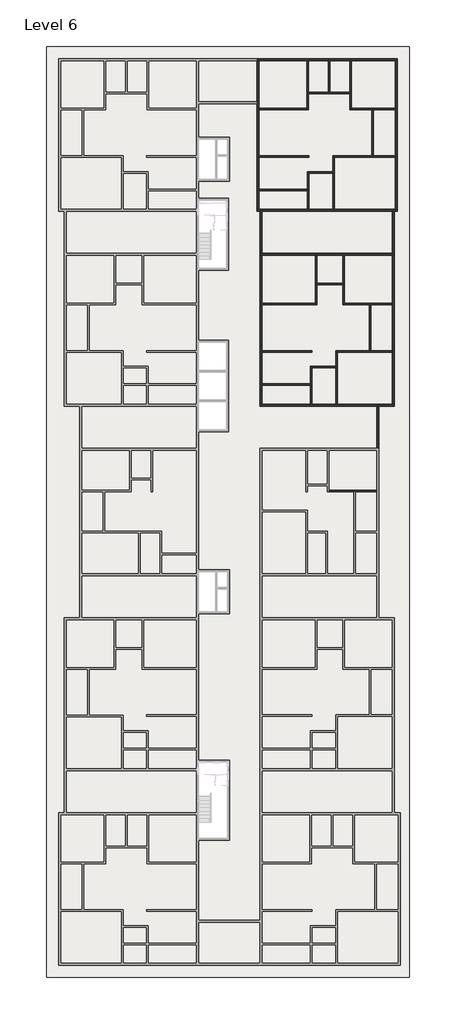
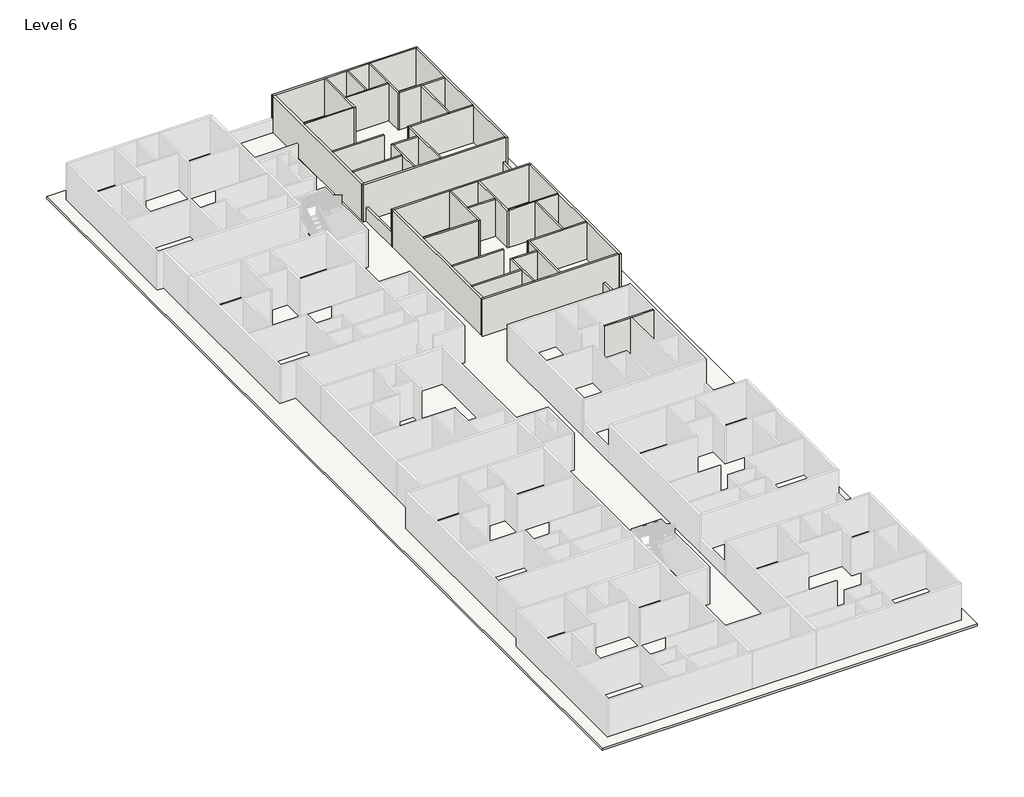
# One storey, part 4 of 8: 37 walls, 1 roof, 1 slab.
"""IFC4 building model written with IfcOpenShell, lengths in millimetres."""

from ifc_helpers import new_model, si_unit, frame, origin, place, context, project, spatial, polyline, outline, extrude, faceted_brep, element, save

model = new_model("IFC4")

# Units and contexts
model_context = context("Model", 3, world=origin())
ifc_project = project(units=[si_unit("LENGTHUNIT", "METRE", prefix="MILLI")], contexts=[model_context])

# Site, building, storey
site = spatial("IfcSite", under=ifc_project)
building = spatial("IfcBuilding", under=site)
storey = spatial("IfcBuildingStorey", under=building, Name="Level 6", Elevation=40474.6172466)

# Roof
placement = place(None, origin())
element("IfcRoof", 1, ObjectType="SLAB", at=placement, inside=storey, context=model_context, shape_type="SweptSolid", body=[
    extrude(outline(polyline([(-15237.9415084, -35021.5344126), (-15237.9415084, 36097.9216096), (12498.9443719, 36097.9216096), (12498.9443719, -35021.5344126), (-15237.9415084, -35021.5344126)]), holes=[polyline([(-3617.4415084, 29152.4900967), (-3617.4415084, 25799.6900967), (-1255.2415084, 25799.6900967), (-1255.2415084, 29152.4900967), (-3617.4415084, 29152.4900967)]), polyline([(-3617.4415084, 24490.1216096), (-3617.4415084, 19003.7216096), (-1331.4415084, 19003.7216096), (-1331.4415084, 24490.1216096), (-3617.4415084, 24490.1216096)]), polyline([(-3617.4415084, 13669.6303368), (-3617.4415084, 6659.2303368), (-1331.4415084, 6659.2303368), (-1331.4415084, 13669.6303368), (-3617.4415084, 13669.6303368)]), polyline([(-3617.4415084, -3882.2751812), (-3617.4415084, -7235.0751812), (-1255.2415084, -7235.0751812), (-1255.2415084, -3882.2751812), (-3617.4415084, -3882.2751812)]), polyline([(-3617.4415084, -18429.9851539), (-3617.4415084, -24525.9851539), (-1229.8415084, -24525.9851539), (-1229.8415084, -18429.9851539), (-3617.4415084, -18429.9851539)])]), frame((0.0, 0.0, 40474.6172466), z_axis=(0.0, 0.0, 1.0), x_axis=(1.0, 0.0, 0.0)), (0.0, 0.0, 1.0), 152.4),
])

# Slab
element("IfcSlab", 2, ObjectType="FLOOR", at=placement, inside=storey, context=model_context, shape_type="SweptSolid", body=[
    extrude(outline(polyline([(-14323.5415084, 35183.5216096), (11584.5443719, 35183.5216096), (11584.5443719, 23499.5216096), (11360.9214687, 23499.5216096), (11360.9214687, 8615.1216096), (10173.4714687, 8615.1216096), (10173.4714687, -7538.7344126), (11360.9214687, -7538.7344126), (11360.9214687, -22423.1344126), (11813.0584916, -22423.1344126), (11813.0584916, -34107.1344126), (11584.5443719, -34107.1344126), (-14323.5415084, -34107.1344126), (-14323.5415084, 35183.5216096)]), holes=[polyline([(-3617.4415084, 29152.4900967), (-3617.4415084, 25799.6900967), (-1255.2415084, 25799.6900967), (-1255.2415084, 29152.4900967), (-3617.4415084, 29152.4900967)]), polyline([(-3617.4415084, 24490.1216096), (-3617.4415084, 19003.7216096), (-1331.4415084, 19003.7216096), (-1331.4415084, 24490.1216096), (-3617.4415084, 24490.1216096)]), polyline([(-3617.4415084, 13669.6303368), (-3617.4415084, 6659.2303368), (-1331.4415084, 6659.2303368), (-1331.4415084, 13669.6303368), (-3617.4415084, 13669.6303368)]), polyline([(-3617.4415084, -3882.2751812), (-3617.4415084, -7235.0751812), (-1255.2415084, -7235.0751812), (-1255.2415084, -3882.2751812), (-3617.4415084, -3882.2751812)]), polyline([(-3617.4415084, -18429.9851539), (-3617.4415084, -24525.9851539), (-1229.8415084, -24525.9851539), (-1229.8415084, -18429.9851539), (-3617.4415084, -18429.9851539)])]), frame((0.0, 0.0, 39865.0172466), z_axis=(0.0, 0.0, 1.0), x_axis=(1.0, 0.0, 0.0)), (0.0, 0.0, 1.0), 609.6),
])

# Walls
element("IfcWall", 3, ObjectType="4.5\"", at=placement, inside=storey, context=model_context, shape_type="Brep", body=[
    faceted_brep([(6363.4714687, 2100.0216096, 40474.6172466), (8282.4584916, 2100.0216096, 40474.6172466), (8396.7584916, 2100.0216096, 40474.6172466), (10021.0714687, 2100.0216096, 40474.6172466), (10021.0714687, 2100.0216096, 43522.6172466), (8396.7584916, 2100.0216096, 43522.6172466), (8282.4584916, 2100.0216096, 43522.6172466), (6363.4714687, 2100.0216096, 43522.6172466), (6363.4714687, 2214.3216096, 40474.6172466), (6363.4714687, 2214.3216096, 43522.6172466), (10021.0714687, 2214.3216096, 43522.6172466), (10021.0714687, 2214.3216096, 40474.6172466)], [[[0, 1, 2, 3, 4, 5, 6, 7]], [[8, 9, 10, 11]], [[3, 2, 1, 0, 8, 11]], [[0, 7, 9, 8]], [[4, 3, 11, 10]], [[7, 6, 5, 4, 10, 9]]]),
])
element("IfcWall", 4, ObjectType="4.5\"", at=placement, inside=storey, context=model_context, shape_type="Brep", body=[
    faceted_brep([(5315.7214687, 20146.7216096, 40474.6172466), (5315.7214687, 16489.1216096, 40474.6172466), (5315.7214687, 16374.8216096, 40474.6172466), (5315.7214687, 16374.8216096, 43522.6172466), (5315.7214687, 16489.1216096, 43522.6172466), (5315.7214687, 20146.7216096, 43522.6172466), (5430.0214687, 20146.7216096, 40474.6172466), (5430.0214687, 20146.7216096, 43522.6172466), (5430.0214687, 18013.1216096, 43522.6172466), (5430.0214687, 17898.8216096, 43522.6172466), (5430.0214687, 16374.8216096, 43522.6172466), (5430.0214687, 16374.8216096, 40474.6172466), (5430.0214687, 17898.8216096, 40474.6172466), (5430.0214687, 18013.1216096, 40474.6172466)], [[[0, 1, 2, 3, 4, 5]], [[6, 7, 8, 9, 10, 11, 12, 13]], [[2, 1, 0, 6, 13, 12, 11]], [[0, 5, 7, 6]], [[3, 2, 11, 10]], [[5, 4, 3, 10, 9, 8, 7]]]),
])
element("IfcWall", 5, ObjectType="4.5\"", at=placement, inside=storey, context=model_context, shape_type="SweptSolid", body=[
    extrude(outline(polyline([(1259.3584916, 16489.1216096), (5315.7214687, 16489.1216096), (5315.7214687, 16374.8216096), (1259.3584916, 16374.8216096), (1259.3584916, 16489.1216096)])), frame((0.0, 0.0, 40474.6172466), z_axis=(0.0, 0.0, 1.0), x_axis=(1.0, 0.0, 0.0)), (0.0, 0.0, 1.0), 3048.0),
])
element("IfcWall", 6, ObjectType="4.5\"", at=placement, inside=storey, context=model_context, shape_type="SweptSolid", body=[
    extrude(outline(polyline([(7436.6214687, 17898.8216096), (5430.0214687, 17898.8216096), (5430.0214687, 18013.1216096), (7436.6214687, 18013.1216096), (7436.6214687, 17898.8216096)])), frame((0.0, 0.0, 40474.6172466), z_axis=(0.0, 0.0, 1.0), x_axis=(1.0, 0.0, 0.0)), (0.0, 0.0, 1.0), 3048.0),
])
element("IfcWall", 7, ObjectType="4.5\"", at=placement, inside=storey, context=model_context, shape_type="Brep", body=[
    faceted_brep([(7436.6214687, 20146.7216096, 40474.6172466), (7436.6214687, 18013.1216096, 40474.6172466), (7436.6214687, 17898.8216096, 40474.6172466), (7436.6214687, 16374.8216096, 40474.6172466), (7436.6214687, 16374.8216096, 43522.6172466), (7436.6214687, 17898.8216096, 43522.6172466), (7436.6214687, 18013.1216096, 43522.6172466), (7436.6214687, 20146.7216096, 43522.6172466), (7550.9214687, 20146.7216096, 40474.6172466), (7550.9214687, 20146.7216096, 43522.6172466), (7550.9214687, 16489.1216096, 43522.6172466), (7550.9214687, 16374.8216096, 43522.6172466), (7550.9214687, 16374.8216096, 40474.6172466), (7550.9214687, 16489.1216096, 40474.6172466)], [[[0, 1, 2, 3, 4, 5, 6, 7]], [[8, 9, 10, 11, 12, 13]], [[3, 2, 1, 0, 8, 13, 12]], [[0, 7, 9, 8]], [[4, 3, 12, 11]], [[7, 6, 5, 4, 11, 10, 9]]]),
])
element("IfcWall", 8, ObjectType="4.5\"", at=placement, inside=storey, context=model_context, shape_type="Brep", body=[
    faceted_brep([(7550.9214687, 16374.8216096, 40474.6172466), (9469.9084916, 16374.8216096, 40474.6172466), (9584.2084916, 16374.8216096, 40474.6172466), (11208.5214687, 16374.8216096, 40474.6172466), (11208.5214687, 16374.8216096, 43522.6172466), (9584.2084916, 16374.8216096, 43522.6172466), (9469.9084916, 16374.8216096, 43522.6172466), (7550.9214687, 16374.8216096, 43522.6172466), (7550.9214687, 16489.1216096, 40474.6172466), (7550.9214687, 16489.1216096, 43522.6172466), (11208.5214687, 16489.1216096, 43522.6172466), (11208.5214687, 16489.1216096, 40474.6172466)], [[[0, 1, 2, 3, 4, 5, 6, 7]], [[8, 9, 10, 11]], [[3, 2, 1, 0, 8, 11]], [[0, 7, 9, 8]], [[4, 3, 11, 10]], [[7, 6, 5, 4, 10, 9]]]),
])
element("IfcWall", 9, ObjectType="4.5\"", at=placement, inside=storey, context=model_context, shape_type="SweptSolid", body=[
    extrude(outline(polyline([(9469.9084916, 12869.6216096), (9469.9084916, 16374.8216096), (9584.2084916, 16374.8216096), (9584.2084916, 12869.6216096), (9469.9084916, 12869.6216096)])), frame((0.0, 0.0, 40474.6172466), z_axis=(0.0, 0.0, 1.0), x_axis=(1.0, 0.0, 0.0)), (0.0, 0.0, 1.0), 3048.0),
])
element("IfcWall", 10, ObjectType="4.5\"", at=placement, inside=storey, context=model_context, shape_type="Brep", body=[
    faceted_brep([(11208.5214687, 12869.6216096, 40474.6172466), (9584.2084916, 12869.6216096, 40474.6172466), (9469.9084916, 12869.6216096, 40474.6172466), (6885.4584916, 12869.6216096, 40474.6172466), (6885.4584916, 12869.6216096, 43522.6172466), (9469.9084916, 12869.6216096, 43522.6172466), (9584.2084916, 12869.6216096, 43522.6172466), (11208.5214687, 12869.6216096, 43522.6172466), (11208.5214687, 12755.3216096, 40474.6172466), (11208.5214687, 12755.3216096, 43522.6172466), (6999.7584916, 12755.3216096, 43522.6172466), (6885.4584916, 12755.3216096, 43522.6172466), (6885.4584916, 12755.3216096, 40474.6172466), (6999.7584916, 12755.3216096, 40474.6172466)], [[[0, 1, 2, 3, 4, 5, 6, 7]], [[8, 9, 10, 11, 12, 13]], [[3, 2, 1, 0, 8, 13, 12]], [[0, 7, 9, 8]], [[4, 3, 12, 11]], [[7, 6, 5, 4, 11, 10, 9]]]),
])
element("IfcWall", 11, ObjectType="4.5\"", at=placement, inside=storey, context=model_context, shape_type="Brep", body=[
    faceted_brep([(6885.4584916, 12755.3216096, 40474.6172466), (6885.4584916, 11663.1216096, 40474.6172466), (6885.4584916, 11548.8216096, 40474.6172466), (6885.4584916, 8767.5216096, 40474.6172466), (6885.4584916, 8767.5216096, 43522.6172466), (6885.4584916, 11548.8216096, 43522.6172466), (6885.4584916, 11663.1216096, 43522.6172466), (6885.4584916, 12755.3216096, 43522.6172466), (6999.7584916, 12755.3216096, 40474.6172466), (6999.7584916, 12755.3216096, 43522.6172466), (6999.7584916, 8767.5216096, 43522.6172466), (6999.7584916, 8767.5216096, 40474.6172466)], [[[0, 1, 2, 3, 4, 5, 6, 7]], [[8, 9, 10, 11]], [[3, 2, 1, 0, 8, 11]], [[0, 7, 9, 8]], [[4, 3, 11, 10]], [[7, 6, 5, 4, 10, 9]]]),
])
element("IfcWall", 12, ObjectType="4.5\"", at=placement, inside=storey, context=model_context, shape_type="Brep", body=[
    faceted_brep([(5056.6584916, 8767.5216096, 40474.6172466), (5056.6584916, 11548.8216096, 40474.6172466), (5056.6584916, 11663.1216096, 40474.6172466), (5056.6584916, 11663.1216096, 43522.6172466), (5056.6584916, 11548.8216096, 43522.6172466), (5056.6584916, 8767.5216096, 43522.6172466), (4942.3584916, 8767.5216096, 40474.6172466), (4942.3584916, 8767.5216096, 43522.6172466), (4942.3584916, 10215.3216096, 43522.6172466), (4942.3584916, 10329.6216096, 43522.6172466), (4942.3584916, 11663.1216096, 43522.6172466), (4942.3584916, 11663.1216096, 40474.6172466), (4942.3584916, 10329.6216096, 40474.6172466), (4942.3584916, 10215.3216096, 40474.6172466)], [[[0, 1, 2, 3, 4, 5]], [[6, 7, 8, 9, 10, 11, 12, 13]], [[2, 1, 0, 6, 13, 12, 11]], [[0, 5, 7, 6]], [[3, 2, 11, 10]], [[5, 4, 3, 10, 9, 8, 7]]]),
])
element("IfcWall", 13, ObjectType="4.5\"", at=placement, inside=storey, context=model_context, shape_type="SweptSolid", body=[
    extrude(outline(polyline([(6885.4584916, 11548.8216096), (5056.6584916, 11548.8216096), (5056.6584916, 11663.1216096), (6885.4584916, 11663.1216096), (6885.4584916, 11548.8216096)])), frame((0.0, 0.0, 40474.6172466), z_axis=(0.0, 0.0, 1.0), x_axis=(1.0, 0.0, 0.0)), (0.0, 0.0, 1.0), 3048.0),
])
element("IfcWall", 14, ObjectType="4.5\"", at=placement, inside=storey, context=model_context, shape_type="SweptSolid", body=[
    extrude(outline(polyline([(4942.3584916, 10215.3216096), (1259.3584916, 10215.3216096), (1259.3584916, 10329.6216096), (4942.3584916, 10329.6216096), (4942.3584916, 10215.3216096)])), frame((0.0, 0.0, 40474.6172466), z_axis=(0.0, 0.0, 1.0), x_axis=(1.0, 0.0, 0.0)), (0.0, 0.0, 1.0), 3048.0),
])
element("IfcWall", 15, ObjectType="4.5\"", at=placement, inside=storey, context=model_context, shape_type="SweptSolid", body=[
    extrude(outline(polyline([(5056.6584916, 12755.3216096), (1259.3584916, 12755.3216096), (1259.3584916, 12869.6216096), (5056.6584916, 12869.6216096), (5056.6584916, 12755.3216096)])), frame((0.0, 0.0, 40474.6172466), z_axis=(0.0, 0.0, 1.0), x_axis=(1.0, 0.0, 0.0)), (0.0, 0.0, 1.0), 3048.0),
])
element("IfcWall", 16, ObjectType="4.5\"", at=placement, inside=storey, context=model_context, shape_type="Brep", body=[
    faceted_brep([(4688.4443719, 35031.1216096, 40474.6172466), (4688.4443719, 31373.5216096, 40474.6172466), (4688.4443719, 31259.2216096, 40474.6172466), (4688.4443719, 31259.2216096, 43522.6172466), (4688.4443719, 31373.5216096, 43522.6172466), (4688.4443719, 35031.1216096, 43522.6172466), (4802.7443719, 35031.1216096, 40474.6172466), (4802.7443719, 35031.1216096, 43522.6172466), (4802.7443719, 32592.7216096, 43522.6172466), (4802.7443719, 32478.4216096, 43522.6172466), (4802.7443719, 31259.2216096, 43522.6172466), (4802.7443719, 31259.2216096, 40474.6172466), (4802.7443719, 32478.4216096, 40474.6172466), (4802.7443719, 32592.7216096, 40474.6172466)], [[[0, 1, 2, 3, 4, 5]], [[6, 7, 8, 9, 10, 11, 12, 13]], [[2, 1, 0, 6, 13, 12, 11]], [[0, 5, 7, 6]], [[3, 2, 11, 10]], [[5, 4, 3, 10, 9, 8, 7]]]),
])
element("IfcWall", 17, ObjectType="4.5\"", at=placement, inside=storey, context=model_context, shape_type="SweptSolid", body=[
    extrude(outline(polyline([(1030.8443719, 31373.5216096), (4688.4443719, 31373.5216096), (4688.4443719, 31259.2216096), (1030.8443719, 31259.2216096), (1030.8443719, 31373.5216096)])), frame((0.0, 0.0, 40474.6172466), z_axis=(0.0, 0.0, 1.0), x_axis=(1.0, 0.0, 0.0)), (0.0, 0.0, 1.0), 3048.0),
])
element("IfcWall", 18, ObjectType="4.5\"", at=placement, inside=storey, context=model_context, shape_type="Brep", body=[
    faceted_brep([(4802.7443719, 32478.4216096, 40474.6172466), (7965.0443719, 32478.4216096, 40474.6172466), (7965.0443719, 32478.4216096, 43522.6172466), (4802.7443719, 32478.4216096, 43522.6172466), (4802.7443719, 32592.7216096, 40474.6172466), (4802.7443719, 32592.7216096, 43522.6172466), (6326.7443719, 32592.7216096, 43522.6172466), (6441.0443719, 32592.7216096, 43522.6172466), (7965.0443719, 32592.7216096, 43522.6172466), (7965.0443719, 32592.7216096, 40474.6172466), (6441.0443719, 32592.7216096, 40474.6172466), (6326.7443719, 32592.7216096, 40474.6172466)], [[[0, 1, 2, 3]], [[4, 5, 6, 7, 8, 9, 10, 11]], [[1, 0, 4, 11, 10, 9]], [[0, 3, 5, 4]], [[2, 1, 9, 8]], [[3, 2, 8, 7, 6, 5]]]),
])
element("IfcWall", 19, ObjectType="4.5\"", at=placement, inside=storey, context=model_context, shape_type="SweptSolid", body=[
    extrude(outline(polyline([(6326.7443719, 32592.7216096), (6326.7443719, 35031.1216096), (6441.0443719, 35031.1216096), (6441.0443719, 32592.7216096), (6326.7443719, 32592.7216096)])), frame((0.0, 0.0, 40474.6172466), z_axis=(0.0, 0.0, 1.0), x_axis=(1.0, 0.0, 0.0)), (0.0, 0.0, 1.0), 3048.0),
])
element("IfcWall", 20, ObjectType="4.5\"", at=placement, inside=storey, context=model_context, shape_type="Brep", body=[
    faceted_brep([(7965.0443719, 35031.1216096, 40474.6172466), (7965.0443719, 32592.7216096, 40474.6172466), (7965.0443719, 32478.4216096, 40474.6172466), (7965.0443719, 31259.2216096, 40474.6172466), (7965.0443719, 31259.2216096, 43522.6172466), (7965.0443719, 32478.4216096, 43522.6172466), (7965.0443719, 32592.7216096, 43522.6172466), (7965.0443719, 35031.1216096, 43522.6172466), (8079.3443719, 35031.1216096, 40474.6172466), (8079.3443719, 35031.1216096, 43522.6172466), (8079.3443719, 31373.5216096, 43522.6172466), (8079.3443719, 31259.2216096, 43522.6172466), (8079.3443719, 31259.2216096, 40474.6172466), (8079.3443719, 31373.5216096, 40474.6172466)], [[[0, 1, 2, 3, 4, 5, 6, 7]], [[8, 9, 10, 11, 12, 13]], [[3, 2, 1, 0, 8, 13, 12]], [[0, 7, 9, 8]], [[4, 3, 12, 11]], [[7, 6, 5, 4, 11, 10, 9]]]),
])
element("IfcWall", 21, ObjectType="4.5\"", at=placement, inside=storey, context=model_context, shape_type="Brep", body=[
    faceted_brep([(8079.3443719, 31259.2216096, 40474.6172466), (9641.4443719, 31259.2216096, 40474.6172466), (9755.7443719, 31259.2216096, 40474.6172466), (11432.1443719, 31259.2216096, 40474.6172466), (11432.1443719, 31259.2216096, 43522.6172466), (9755.7443719, 31259.2216096, 43522.6172466), (9641.4443719, 31259.2216096, 43522.6172466), (8079.3443719, 31259.2216096, 43522.6172466), (8079.3443719, 31373.5216096, 40474.6172466), (8079.3443719, 31373.5216096, 43522.6172466), (11432.1443719, 31373.5216096, 43522.6172466), (11432.1443719, 31373.5216096, 40474.6172466)], [[[0, 1, 2, 3, 4, 5, 6, 7]], [[8, 9, 10, 11]], [[3, 2, 1, 0, 8, 11]], [[0, 7, 9, 8]], [[4, 3, 11, 10]], [[7, 6, 5, 4, 10, 9]]]),
])
element("IfcWall", 22, ObjectType="4.5\"", at=placement, inside=storey, context=model_context, shape_type="SweptSolid", body=[
    extrude(outline(polyline([(9641.4443719, 27754.0216096), (9641.4443719, 31259.2216096), (9755.7443719, 31259.2216096), (9755.7443719, 27754.0216096), (9641.4443719, 27754.0216096)])), frame((0.0, 0.0, 40474.6172466), z_axis=(0.0, 0.0, 1.0), x_axis=(1.0, 0.0, 0.0)), (0.0, 0.0, 1.0), 3048.0),
])
element("IfcWall", 23, ObjectType="4.5\"", at=placement, inside=storey, context=model_context, shape_type="Brep", body=[
    faceted_brep([(11432.1443719, 27754.0216096, 40474.6172466), (9755.7443719, 27754.0216096, 40474.6172466), (9641.4443719, 27754.0216096, 40474.6172466), (6656.9443719, 27754.0216096, 40474.6172466), (6656.9443719, 27754.0216096, 43522.6172466), (9641.4443719, 27754.0216096, 43522.6172466), (9755.7443719, 27754.0216096, 43522.6172466), (11432.1443719, 27754.0216096, 43522.6172466), (11432.1443719, 27639.7216096, 40474.6172466), (11432.1443719, 27639.7216096, 43522.6172466), (6771.2443719, 27639.7216096, 43522.6172466), (6656.9443719, 27639.7216096, 43522.6172466), (6656.9443719, 27639.7216096, 40474.6172466), (6771.2443719, 27639.7216096, 40474.6172466)], [[[0, 1, 2, 3, 4, 5, 6, 7]], [[8, 9, 10, 11, 12, 13]], [[3, 2, 1, 0, 8, 13, 12]], [[0, 7, 9, 8]], [[4, 3, 12, 11]], [[7, 6, 5, 4, 11, 10, 9]]]),
])
element("IfcWall", 24, ObjectType="4.5\"", at=placement, inside=storey, context=model_context, shape_type="Brep", body=[
    faceted_brep([(6656.9443719, 27639.7216096, 40474.6172466), (6656.9443719, 26547.5216096, 40474.6172466), (6656.9443719, 26433.2216096, 40474.6172466), (6656.9443719, 23651.9216096, 40474.6172466), (6656.9443719, 23651.9216096, 43522.6172466), (6656.9443719, 26433.2216096, 43522.6172466), (6656.9443719, 26547.5216096, 43522.6172466), (6656.9443719, 27639.7216096, 43522.6172466), (6771.2443719, 27639.7216096, 40474.6172466), (6771.2443719, 27639.7216096, 43522.6172466), (6771.2443719, 23651.9216096, 43522.6172466), (6771.2443719, 23651.9216096, 40474.6172466)], [[[0, 1, 2, 3, 4, 5, 6, 7]], [[8, 9, 10, 11]], [[3, 2, 1, 0, 8, 11]], [[0, 7, 9, 8]], [[4, 3, 11, 10]], [[7, 6, 5, 4, 10, 9]]]),
])
element("IfcWall", 25, ObjectType="4.5\"", at=placement, inside=storey, context=model_context, shape_type="SweptSolid", body=[
    extrude(outline(polyline([(4713.8443719, 25099.7216096), (1030.8443719, 25099.7216096), (1030.8443719, 25214.0216096), (4713.8443719, 25214.0216096), (4713.8443719, 25099.7216096)])), frame((0.0, 0.0, 40474.6172466), z_axis=(0.0, 0.0, 1.0), x_axis=(1.0, 0.0, 0.0)), (0.0, 0.0, 1.0), 3048.0),
])
element("IfcWall", 26, ObjectType="4.5\"", at=placement, inside=storey, context=model_context, shape_type="Brep", body=[
    faceted_brep([(4828.1443719, 23651.9216096, 40474.6172466), (4828.1443719, 26433.2216096, 40474.6172466), (4828.1443719, 26547.5216096, 40474.6172466), (4828.1443719, 26547.5216096, 43522.6172466), (4828.1443719, 26433.2216096, 43522.6172466), (4828.1443719, 23651.9216096, 43522.6172466), (4713.8443719, 23651.9216096, 40474.6172466), (4713.8443719, 23651.9216096, 43522.6172466), (4713.8443719, 25099.7216096, 43522.6172466), (4713.8443719, 25214.0216096, 43522.6172466), (4713.8443719, 26547.5216096, 43522.6172466), (4713.8443719, 26547.5216096, 40474.6172466), (4713.8443719, 25214.0216096, 40474.6172466), (4713.8443719, 25099.7216096, 40474.6172466)], [[[0, 1, 2, 3, 4, 5]], [[6, 7, 8, 9, 10, 11, 12, 13]], [[2, 1, 0, 6, 13, 12, 11]], [[0, 5, 7, 6]], [[3, 2, 11, 10]], [[5, 4, 3, 10, 9, 8, 7]]]),
])
element("IfcWall", 27, ObjectType="4.5\"", at=placement, inside=storey, context=model_context, shape_type="SweptSolid", body=[
    extrude(outline(polyline([(6656.9443719, 26433.2216096), (4828.1443719, 26433.2216096), (4828.1443719, 26547.5216096), (6656.9443719, 26547.5216096), (6656.9443719, 26433.2216096)])), frame((0.0, 0.0, 40474.6172466), z_axis=(0.0, 0.0, 1.0), x_axis=(1.0, 0.0, 0.0)), (0.0, 0.0, 1.0), 3048.0),
])
element("IfcWall", 28, ObjectType="4.5\"", at=placement, inside=storey, context=model_context, shape_type="SweptSolid", body=[
    extrude(outline(polyline([(4828.1443719, 27639.7216096), (1030.8443719, 27639.7216096), (1030.8443719, 27754.0216096), (4828.1443719, 27754.0216096), (4828.1443719, 27639.7216096)])), frame((0.0, 0.0, 40474.6172466), z_axis=(0.0, 0.0, 1.0), x_axis=(1.0, 0.0, 0.0)), (0.0, 0.0, 1.0), 3048.0),
])
element("IfcWall", 29, ObjectType="6\"", at=placement, inside=storey, context=model_context, shape_type="Brep", body=[
    faceted_brep([(1106.9584916, 20146.7216096, 43522.6172466), (1106.9584916, 20146.7216096, 40474.6172466), (1259.3584916, 20146.7216096, 40474.6172466), (5315.7214687, 20146.7216096, 40474.6172466), (5430.0214687, 20146.7216096, 40474.6172466), (7436.6214687, 20146.7216096, 40474.6172466), (7550.9214687, 20146.7216096, 40474.6172466), (11208.5214687, 20146.7216096, 40474.6172466), (11360.9214687, 20146.7216096, 40474.6172466), (11360.9214687, 20146.7216096, 43522.6172466), (11208.5214687, 20146.7216096, 43522.6172466), (7550.9214687, 20146.7216096, 43522.6172466), (7436.6214687, 20146.7216096, 43522.6172466), (5430.0214687, 20146.7216096, 43522.6172466), (5315.7214687, 20146.7216096, 43522.6172466), (1259.3584916, 20146.7216096, 43522.6172466), (1106.9584916, 20299.1216096, 40474.6172466), (1106.9584916, 20299.1216096, 41693.8172466), (1106.9584916, 20299.1216096, 43522.6172466), (11360.9214687, 20299.1216096, 43522.6172466), (11360.9214687, 20299.1216096, 41693.8172466), (11360.9214687, 20299.1216096, 40474.6172466), (11208.5214687, 20299.1216096, 40474.6172466), (1259.3584916, 20299.1216096, 40474.6172466)], [[[0, 1, 2, 3, 4, 5, 6, 7, 8, 9, 10, 11, 12, 13, 14, 15]], [[16, 17, 18, 19, 20, 21, 22, 23]], [[8, 7, 6, 5, 4, 3, 2, 1, 16, 23, 22, 21]], [[0, 18, 17, 16, 1]], [[8, 21, 20, 19, 9]], [[0, 15, 14, 13, 12, 11, 10, 9, 19, 18]]]),
])
element("IfcWall", 30, ObjectType="6\"", at=placement, inside=storey, context=model_context, shape_type="Brep", body=[
    faceted_brep([(11208.5214687, 20146.7216096, 43522.6172466), (11208.5214687, 20146.7216096, 40474.6172466), (11208.5214687, 16489.1216096, 40474.6172466), (11208.5214687, 16374.8216096, 40474.6172466), (11208.5214687, 12869.6216096, 40474.6172466), (11208.5214687, 12755.3216096, 40474.6172466), (11208.5214687, 8767.5216096, 40474.6172466), (11208.5214687, 8615.1216096, 40474.6172466), (11208.5214687, 8615.1216096, 43522.6172466), (11208.5214687, 8767.5216096, 43522.6172466), (11208.5214687, 12755.3216096, 43522.6172466), (11208.5214687, 12869.6216096, 43522.6172466), (11208.5214687, 16374.8216096, 43522.6172466), (11208.5214687, 16489.1216096, 43522.6172466), (11360.9214687, 20146.7216096, 40474.6172466), (11360.9214687, 20146.7216096, 43522.6172466), (11360.9214687, 8615.1216096, 43522.6172466), (11360.9214687, 8615.1216096, 40474.6172466)], [[[0, 1, 2, 3, 4, 5, 6, 7, 8, 9, 10, 11, 12, 13]], [[14, 15, 16, 17]], [[7, 6, 5, 4, 3, 2, 1, 14, 17]], [[8, 7, 17, 16]], [[0, 15, 14, 1]], [[0, 13, 12, 11, 10, 9, 8, 16, 15]]]),
])
element("IfcWall", 31, ObjectType="6\"", at=placement, inside=storey, context=model_context, shape_type="Brep", body=[
    faceted_brep([(11208.5214687, 8767.5216096, 40474.6172466), (6999.7584916, 8767.5216096, 40474.6172466), (6885.4584916, 8767.5216096, 40474.6172466), (5056.6584916, 8767.5216096, 40474.6172466), (4942.3584916, 8767.5216096, 40474.6172466), (1259.3584916, 8767.5216096, 40474.6172466), (1106.9584916, 8767.5216096, 40474.6172466), (1106.9584916, 8767.5216096, 43522.6172466), (1259.3584916, 8767.5216096, 43522.6172466), (4942.3584916, 8767.5216096, 43522.6172466), (5056.6584916, 8767.5216096, 43522.6172466), (6885.4584916, 8767.5216096, 43522.6172466), (6999.7584916, 8767.5216096, 43522.6172466), (11208.5214687, 8767.5216096, 43522.6172466), (11208.5214687, 8615.1216096, 40474.6172466), (11208.5214687, 8615.1216096, 43522.6172466), (1106.9584916, 8615.1216096, 43522.6172466), (1106.9584916, 8615.1216096, 40474.6172466), (10021.0714687, 8615.1216096, 40474.6172466), (10173.4714687, 8615.1216096, 40474.6172466)], [[[0, 1, 2, 3, 4, 5, 6, 7, 8, 9, 10, 11, 12, 13]], [[14, 15, 16, 17, 18, 19]], [[6, 5, 4, 3, 2, 1, 0, 14, 19, 18, 17]], [[0, 13, 15, 14]], [[7, 6, 17, 16]], [[13, 12, 11, 10, 9, 8, 7, 16, 15]]]),
])
element("IfcWall", 32, ObjectType="6\"", at=placement, inside=storey, context=model_context, shape_type="Brep", body=[
    faceted_brep([(1259.3584916, 8767.5216096, 40474.6172466), (1259.3584916, 10215.3216096, 40474.6172466), (1259.3584916, 10329.6216096, 40474.6172466), (1259.3584916, 12755.3216096, 40474.6172466), (1259.3584916, 12869.6216096, 40474.6172466), (1259.3584916, 16374.8216096, 40474.6172466), (1259.3584916, 16489.1216096, 40474.6172466), (1259.3584916, 20146.7216096, 40474.6172466), (1259.3584916, 20146.7216096, 43522.6172466), (1259.3584916, 16489.1216096, 43522.6172466), (1259.3584916, 16374.8216096, 43522.6172466), (1259.3584916, 12869.6216096, 43522.6172466), (1259.3584916, 12755.3216096, 43522.6172466), (1259.3584916, 10329.6216096, 43522.6172466), (1259.3584916, 10215.3216096, 43522.6172466), (1259.3584916, 8767.5216096, 43522.6172466), (1106.9584916, 8767.5216096, 40474.6172466), (1106.9584916, 8767.5216096, 43522.6172466), (1106.9584916, 20146.7216096, 43522.6172466), (1106.9584916, 20146.7216096, 40474.6172466)], [[[0, 1, 2, 3, 4, 5, 6, 7, 8, 9, 10, 11, 12, 13, 14, 15]], [[16, 17, 18, 19]], [[7, 6, 5, 4, 3, 2, 1, 0, 16, 19]], [[0, 15, 17, 16]], [[7, 19, 18, 8]], [[15, 14, 13, 12, 11, 10, 9, 8, 18, 17]]]),
])
element("IfcWall", 33, ObjectType="6\"", at=placement, inside=storey, context=model_context, shape_type="Brep", body=[
    faceted_brep([(878.4443719, 35031.1216096, 43522.6172466), (878.4443719, 35031.1216096, 40474.6172466), (1030.8443719, 35031.1216096, 40474.6172466), (4688.4443719, 35031.1216096, 40474.6172466), (4802.7443719, 35031.1216096, 40474.6172466), (6326.7443719, 35031.1216096, 40474.6172466), (6441.0443719, 35031.1216096, 40474.6172466), (7965.0443719, 35031.1216096, 40474.6172466), (8079.3443719, 35031.1216096, 40474.6172466), (11432.1443719, 35031.1216096, 40474.6172466), (11584.5443719, 35031.1216096, 40474.6172466), (11584.5443719, 35031.1216096, 43522.6172466), (11432.1443719, 35031.1216096, 43522.6172466), (8079.3443719, 35031.1216096, 43522.6172466), (7965.0443719, 35031.1216096, 43522.6172466), (6441.0443719, 35031.1216096, 43522.6172466), (6326.7443719, 35031.1216096, 43522.6172466), (4802.7443719, 35031.1216096, 43522.6172466), (4688.4443719, 35031.1216096, 43522.6172466), (1030.8443719, 35031.1216096, 43522.6172466), (878.4443719, 35183.5216096, 40474.6172466), (878.4443719, 35183.5216096, 43522.6172466), (11584.5443719, 35183.5216096, 43522.6172466), (11584.5443719, 35183.5216096, 40474.6172466)], [[[0, 1, 2, 3, 4, 5, 6, 7, 8, 9, 10, 11, 12, 13, 14, 15, 16, 17, 18, 19]], [[20, 21, 22, 23]], [[10, 9, 8, 7, 6, 5, 4, 3, 2, 1, 20, 23]], [[11, 10, 23, 22]], [[0, 21, 20, 1]], [[0, 19, 18, 17, 16, 15, 14, 13, 12, 11, 22, 21]]]),
])
element("IfcWall", 34, ObjectType="6\"", at=placement, inside=storey, context=model_context, shape_type="Brep", body=[
    faceted_brep([(11432.1443719, 35031.1216096, 40474.6172466), (11432.1443719, 31373.5216096, 40474.6172466), (11432.1443719, 31259.2216096, 40474.6172466), (11432.1443719, 27754.0216096, 40474.6172466), (11432.1443719, 27639.7216096, 40474.6172466), (11432.1443719, 23651.9216096, 40474.6172466), (11432.1443719, 23499.5216096, 40474.6172466), (11432.1443719, 23499.5216096, 43522.6172466), (11432.1443719, 23651.9216096, 43522.6172466), (11432.1443719, 27639.7216096, 43522.6172466), (11432.1443719, 27754.0216096, 43522.6172466), (11432.1443719, 31259.2216096, 43522.6172466), (11432.1443719, 31373.5216096, 43522.6172466), (11432.1443719, 35031.1216096, 43522.6172466), (11584.5443719, 35031.1216096, 40474.6172466), (11584.5443719, 35031.1216096, 43522.6172466), (11584.5443719, 23499.5216096, 43522.6172466), (11584.5443719, 23499.5216096, 40474.6172466)], [[[0, 1, 2, 3, 4, 5, 6, 7, 8, 9, 10, 11, 12, 13]], [[14, 15, 16, 17]], [[6, 5, 4, 3, 2, 1, 0, 14, 17]], [[0, 13, 15, 14]], [[7, 6, 17, 16]], [[13, 12, 11, 10, 9, 8, 7, 16, 15]]]),
])
element("IfcWall", 35, ObjectType="6\"", at=placement, inside=storey, context=model_context, shape_type="Brep", body=[
    faceted_brep([(11432.1443719, 23651.9216096, 40474.6172466), (6771.2443719, 23651.9216096, 40474.6172466), (6656.9443719, 23651.9216096, 40474.6172466), (4828.1443719, 23651.9216096, 40474.6172466), (4713.8443719, 23651.9216096, 40474.6172466), (1030.8443719, 23651.9216096, 40474.6172466), (878.4443719, 23651.9216096, 40474.6172466), (878.4443719, 23651.9216096, 43522.6172466), (1030.8443719, 23651.9216096, 43522.6172466), (4713.8443719, 23651.9216096, 43522.6172466), (4828.1443719, 23651.9216096, 43522.6172466), (6656.9443719, 23651.9216096, 43522.6172466), (6771.2443719, 23651.9216096, 43522.6172466), (11432.1443719, 23651.9216096, 43522.6172466), (11432.1443719, 23499.5216096, 40474.6172466), (11432.1443719, 23499.5216096, 43522.6172466), (878.4443719, 23499.5216096, 43522.6172466), (878.4443719, 23499.5216096, 40474.6172466), (1106.9584916, 23499.5216096, 40474.6172466), (1259.3584916, 23499.5216096, 40474.6172466), (11208.5214687, 23499.5216096, 40474.6172466), (11360.9214687, 23499.5216096, 40474.6172466)], [[[0, 1, 2, 3, 4, 5, 6, 7, 8, 9, 10, 11, 12, 13]], [[14, 15, 16, 17, 18, 19, 20, 21]], [[6, 5, 4, 3, 2, 1, 0, 14, 21, 20, 19, 18, 17]], [[0, 13, 15, 14]], [[7, 6, 17, 16]], [[13, 12, 11, 10, 9, 8, 7, 16, 15]]]),
])
element("IfcWall", 36, ObjectType="6\"", at=placement, inside=storey, context=model_context, shape_type="Brep", body=[
    faceted_brep([(1030.8443719, 23651.9216096, 40474.6172466), (1030.8443719, 25099.7216096, 40474.6172466), (1030.8443719, 25214.0216096, 40474.6172466), (1030.8443719, 27639.7216096, 40474.6172466), (1030.8443719, 27754.0216096, 40474.6172466), (1030.8443719, 31259.2216096, 40474.6172466), (1030.8443719, 31373.5216096, 40474.6172466), (1030.8443719, 35031.1216096, 40474.6172466), (1030.8443719, 35031.1216096, 43522.6172466), (1030.8443719, 31373.5216096, 43522.6172466), (1030.8443719, 31259.2216096, 43522.6172466), (1030.8443719, 27754.0216096, 43522.6172466), (1030.8443719, 27639.7216096, 43522.6172466), (1030.8443719, 25214.0216096, 43522.6172466), (1030.8443719, 25099.7216096, 43522.6172466), (1030.8443719, 23651.9216096, 43522.6172466), (878.4443719, 23651.9216096, 40474.6172466), (878.4443719, 23651.9216096, 43522.6172466), (878.4443719, 35031.1216096, 43522.6172466), (878.4443719, 35031.1216096, 40474.6172466), (878.4443719, 31897.3197155, 40474.6172466), (878.4443719, 31744.9197155, 40474.6172466)], [[[0, 1, 2, 3, 4, 5, 6, 7, 8, 9, 10, 11, 12, 13, 14, 15]], [[16, 17, 18, 19, 20, 21]], [[7, 6, 5, 4, 3, 2, 1, 0, 16, 21, 20, 19]], [[0, 15, 17, 16]], [[7, 19, 18, 8]], [[15, 14, 13, 12, 11, 10, 9, 8, 18, 17]]]),
])
element("IfcWall", 37, ObjectType="6\" 2", at=placement, inside=storey, context=model_context, shape_type="SweptSolid", body=[
    extrude(outline(polyline([(1106.9584916, 20299.1216096), (1106.9584916, 23499.5216096), (1259.3584916, 23499.5216096), (1259.3584916, 20299.1216096), (1106.9584916, 20299.1216096)])), frame((0.0, 0.0, 40474.6172466), z_axis=(0.0, 0.0, 1.0), x_axis=(1.0, 0.0, 0.0)), (0.0, 0.0, 1.0), 1219.2),
])
element("IfcWall", 38, ObjectType="6\" 2", at=placement, inside=storey, context=model_context, shape_type="SweptSolid", body=[
    extrude(outline(polyline([(11208.5214687, 20299.1216096), (11208.5214687, 23499.5216096), (11360.9214687, 23499.5216096), (11360.9214687, 20299.1216096), (11208.5214687, 20299.1216096)])), frame((0.0, 0.0, 40474.6172466), z_axis=(0.0, 0.0, 1.0), x_axis=(1.0, 0.0, 0.0)), (0.0, 0.0, 1.0), 1219.2),
])
element("IfcWall", 39, ObjectType="6\" 2", at=placement, inside=storey, context=model_context, shape_type="SweptSolid", body=[
    extrude(outline(polyline([(10021.0714687, 5414.7216096), (10021.0714687, 8615.1216096), (10173.4714687, 8615.1216096), (10173.4714687, 5414.7216096), (10021.0714687, 5414.7216096)])), frame((0.0, 0.0, 40474.6172466), z_axis=(0.0, 0.0, 1.0), x_axis=(1.0, 0.0, 0.0)), (0.0, 0.0, 1.0), 1219.2),
])

save(model, "model.ifc")

# Revit data of these elements
# Type "SLAB"
#   Assembly Code = "B1020"
#   Layers, outside or top first: 0' - 6" "Damp-proofing" (function 1)
# Type "FLOOR"
#   Assembly Code = "B1010"
#   Function = 0
#   Layers, outside or top first: 2' - 0" "Tile, Porcelain, 4in" (function 1)
# Type "4.5\""
#   Assembly Code = "B2010"
#   Layers, outside or top first: 0' - 4 1/2" "WALLS" (function 1)
# Type "6\""
#   Assembly Code = "B2010"
#   Layers, outside or top first: 0' - 6" "WALLS" (function 1)
# Type "6\" 2"
#   Assembly Code = "B2010"
#   Layers, outside or top first: 0' - 6" "4'" (function 1)
# Element 1 (IfcRoof, "SLAB")
#   built-in parameter 1001705 = 133.291 (stored number, unit not read)
#   built-in parameter 1001710 = 33615
#   Phase Created = New Construction
#   Materials on its faces: "Damp-proofing"
# Element 2 (IfcSlab, "FLOOR")
#   built-in parameter 1001955 = 3.14159 (stored number, unit not read)
#   Height Offset From Level = 0' - 0"
#   Phase Created = New Construction
#   Materials on its faces: "Tile, Porcelain, 4in"
# Elements 3, 4, 5, 6, 7, 8, 9, 10, 11, 12, 13, 14, 15, 16, 17, 18, 19, 20, 21, 22, 23, 24, 25, 26, 27, 28 (IfcWall, "4.5\"")
#   Top Offset = 0' - 0"
#   Base Offset = 0' - 0"
#   Unconnected Height = 10' - 0"
#   wall height = 10' - 0"
#   Phase Created = New Construction
#   Base Constraint = Level 6
#   Materials on its faces: "WALLS"
# Elements 29, 30, 31, 32, 33, 34, 35, 36 (IfcWall, "6\"")
#   Top Offset = 0' - 0"
#   Base Offset = 0' - 0"
#   Unconnected Height = 10' - 0"
#   wall height = 10' - 0"
#   Phase Created = New Construction
#   Base Constraint = Level 6
#   Materials on its faces: "WALLS"
# Elements 37, 38, 39 (IfcWall, "6\" 2")
#   Top Offset = 0' - 0"
#   Base Offset = 0' - 0"
#   Unconnected Height = 4' - 0"
#   wall height = 4' - 0"
#   Phase Created = New Construction
#   Base Constraint = Level 6
#   Materials on its faces: "4'"
# Materials
#   "Damp-proofing": class "Generic", colour RGB 127 127 127, transparency 0, Description = "Damp-proofing", Cost = 0
#   "Tile, Porcelain, 4in": class "Generic", colour RGB 89 87 158, transparency 0, Description = "Porcelain tile, 4\", white", Cost = 0
#   "WALLS": class "Generic", colour RGB 120 120 120, transparency 0, Cost = 0
#   "4'": class "Generic", colour RGB 120 120 120, transparency 0, Cost = 0
